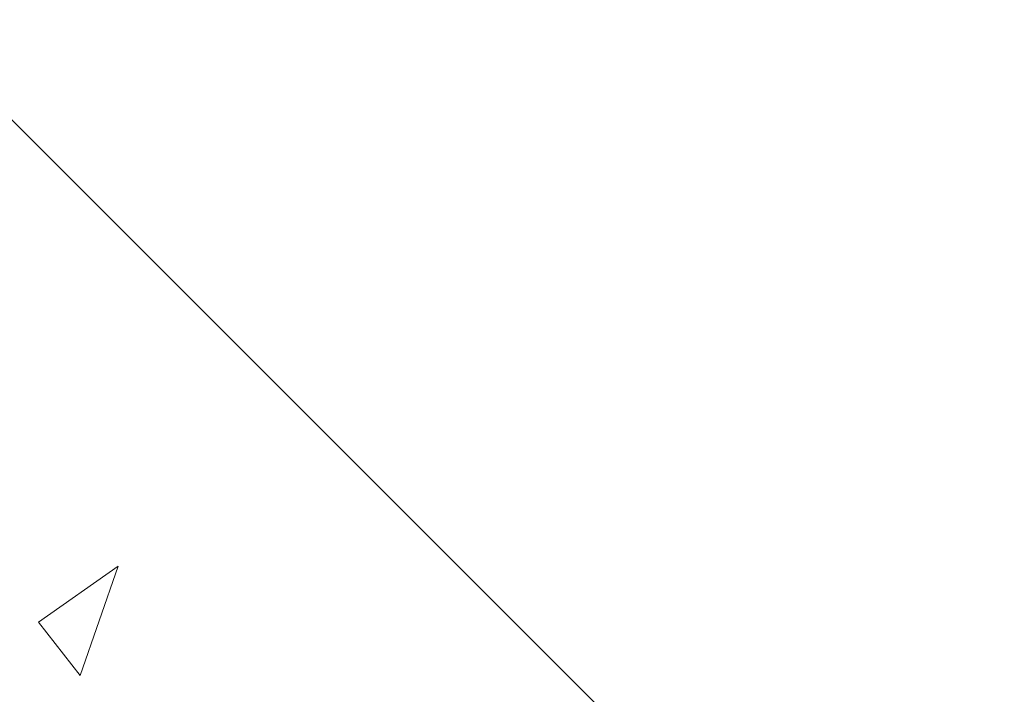
# Model space of a CAD drawing. Units: inches. Extents: x 459864 to 460310, y 324185 to 324787.
# Tile 13 of 112: x 460072.714 to 460075.971, y 324238.89 to 324241.122. Entities that reach past the tile are written whole.
import ezdxf

# ---------------------------------------------------------------- set-up
doc = ezdxf.new("R2010")
doc.units = ezdxf.units.IN
doc.layers.add('A-ANNO-DIMS', color=2, linetype='Continuous', lineweight=18)
doc.layers.add('L-HRDS', color=9, linetype='Continuous', lineweight=18)
doc.styles.get("Standard").update_dxf_attribs({"font": 'arial.ttf'})
doc.dimstyles.new('ISO-25', dxfattribs={"dimtxt": 6, "dimasz": 2.5, "dimexe": 1.25, "dimexo": 0.625, "dimtad": 1, "dimdec": 1, "dimlunit": 3, "dimtxsty": 'Standard', "dimcen": 2.5, "dimadec": 0, "dimazin": 0, "dimtfac": 1, "dimtdec": 1, "dimtmove": 0, "dimatfit": 3, "dimfxl": 1, "dimarcsym": 0})

# ---------------------------------------------------------------- blocks, each defined once
blk = doc.blocks.new('Stepping Stone - hexagonal')
for p, q in [((9.0601, 4.2016), (3.1951, 10.0666)), ((4.3331, 7.0526), (3.8951, 6.7436)), ((4.1251, 6.4496), (4.3331, 7.0526)), ((3.8951, 6.7436), (4.1251, 6.4496))]:
    blk.add_line(p, q)
blk = doc.blocks.new('*D36')
at = {"layer": 'A-ANNO-DIMS', "color": 0, "lineweight": -2, "transparency": 16777216}
for p, q in [((460063.8613, 324228.4828), (460063.8613, 324226.0557)), ((460075.8757, 324228.4828), (460075.8757, 324226.0557)), ((460066.3613, 324227.3057), (460073.3757, 324227.3057)), ((460075.8757, 324227.3057), (460126.0214, 324227.3057))]:
    blk.add_line(p, q, dxfattribs=at)
at = {"layer": 'A-ANNO-DIMS', "color": 0, "transparency": 16777216}
for points in [[(460066.3613, 324227.7223), (460066.3613, 324226.889), (460063.8613, 324227.3057)], [(460073.3757, 324227.7223), (460073.3757, 324226.889), (460075.8757, 324227.3057)]]:
    blk.add_solid(points, dxfattribs=at)
at = {"layer": 'Defpoints', "color": 0, "transparency": 16777216}
for p in [(460063.8613, 324229.1078), (460075.8757, 324229.1078), (460075.8757, 324227.3057)]:
    blk.add_point(p, dxfattribs=at)
at = {"layer": 'A-ANNO-DIMS', "color": 0, "transparency": 16777216, "insert": (460102.1986, 324230.9941), "char_height": 6, "attachment_point": 5}
blk.add_mtext('PAVER 1\'-0"', dxfattribs=at)

msp = doc.modelspace()

# ---------------------------------------------------------------- block references
at = {"layer": 'L-HRDS', "xscale": 0.6, "yscale": 0.6}
msp.add_blockref('Stepping Stone - hexagonal', (460070.4397, 324235.0823), dxfattribs=at)

# ---------------------------------------------------------------- dimensions: what is measured, and where the dimension line sits
at = {"layer": 'A-ANNO-DIMS'}
dim = msp.add_linear_dim(base=(460075.8757, 324227.3057), p1=(460063.8613, 324229.1078), p2=(460075.8757, 324229.1078), text='PAVER <>', dimstyle='ISO-25', override={"dimdec": 1, "dimlfac": 1, "dimrnd": 0, "dimzin": 1, "dimdsep": 46, "dimlunit": 4, "dimfrac": 2}, dxfattribs=at)
dim.commit()
dim.dimension.update_dxf_attribs({"geometry": '*D36', "text_midpoint": (460102.1986, 324230.9941)})

doc.saveas('drawing.dxf')
